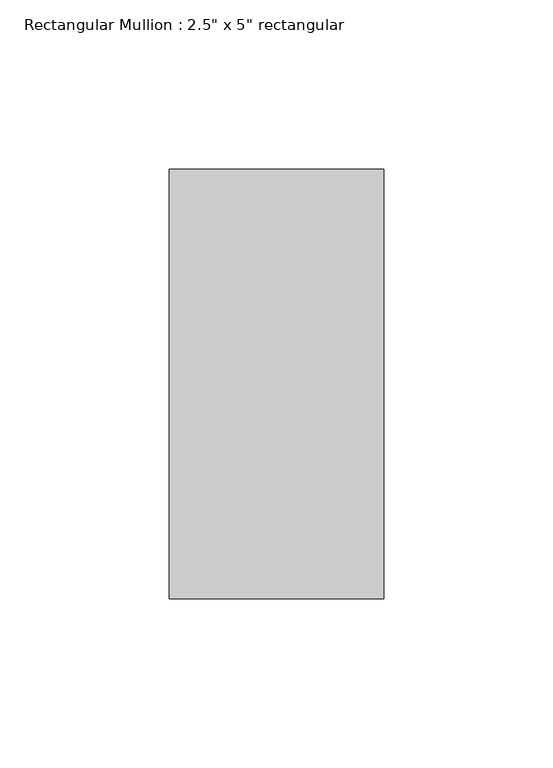
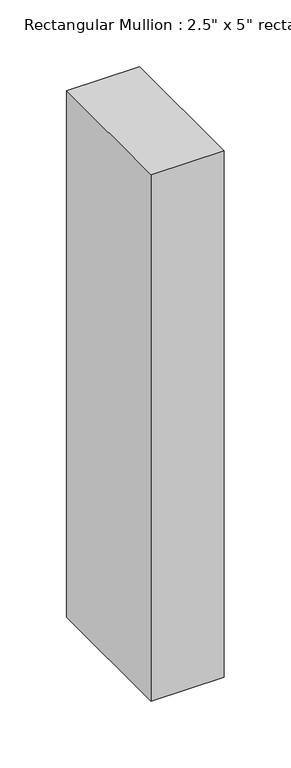
"""IFC4 building model written with IfcOpenShell, lengths in millimetres: member geometry."""

from ifc_helpers import new_model, si_unit, frame, origin, place, context, project, spatial, polyline, outline, extrude, source, transform, mapped, element, save


def member_323df77c(model_context):
    return source(origin(), model_context, "Body", "SweptSolid", [
        extrude(outline(polyline([(31.75, 63.5), (31.75, -63.5), (-31.75, -63.5), (-31.75, 63.5), (31.75, 63.5)])), frame((0.0, 0.0, -482.6), z_axis=(0.0, 0.0, 1.0), x_axis=(1.0, 0.0, 0.0)), (0.0, 0.0, 1.0), 482.6),
    ])


if __name__ == "__main__":
    model = new_model("IFC4")
    model_context = context("Model", 3, world=origin())
    ifc_project = project(units=[si_unit("LENGTHUNIT", "METRE", prefix="MILLI")], contexts=[model_context])
    site = spatial("IfcSite", under=ifc_project)
    building = spatial("IfcBuilding", under=site)
    placement = place(None, origin())
    member_shape = member_323df77c(model_context)
    element("IfcMember", 1, ObjectType="Rectangular Mullion : 2.5\" x 5\" rectangular", at=placement, inside=building, context=model_context, shape_type="MappedRepresentation", body=[
        mapped(member_shape, transform((0.0, 0.0, 0.0), x_axis=(1.0, 0.0, 0.0), y_axis=(0.0, 1.0, 0.0), z_axis=(0.0, 0.0, 1.0))),
    ])
    save(model, "model.ifc")

# Revit data of these elements
# Type "Rectangular Mullion : 2.5\" x 5\" rectangular"
#   built-in parameter 1007304 = 0.416667 (stored number, unit not read)
#   built-in parameter 1007301 = 0.104167 (stored number, unit not read)
#   built-in parameter 1007300 = 0.104167 (stored number, unit not read)
